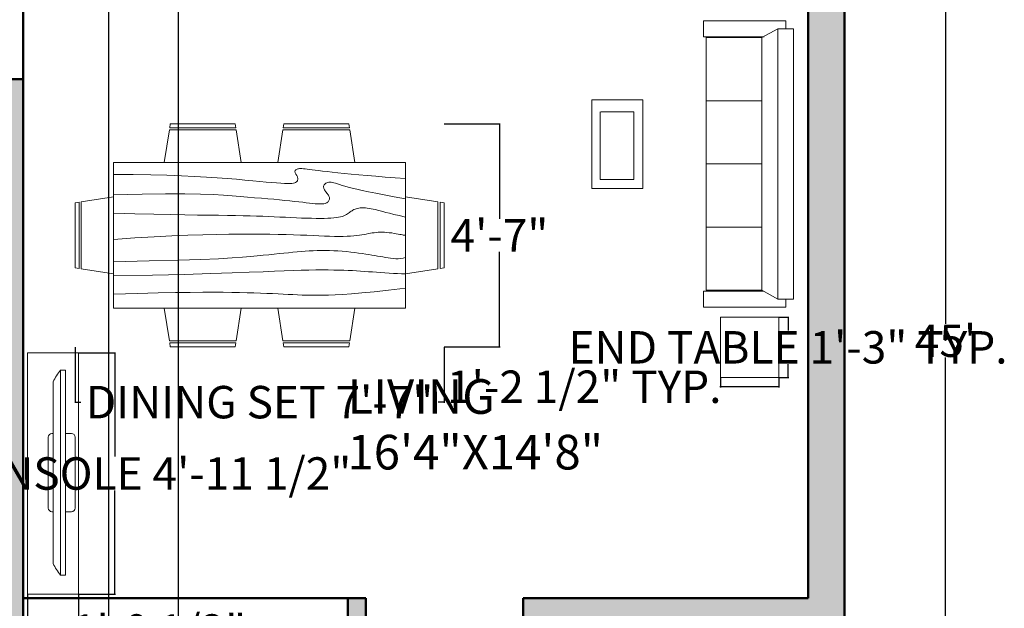
# Model space of a CAD drawing. Units: inches. Extents: x 22042254 to 25404563, y 17568978 to 17626777.
# Tile 42 of 45: x 22179940 to 22180183, y 17626402 to 17626547. Entities that reach past the tile are written whole.
import ezdxf

# ---------------------------------------------------------------- set-up
doc = ezdxf.new("R2010")
doc.units = ezdxf.units.IN
doc.header["$MEASUREMENT"] = 0
for name, color, linetype, lineweight in [('A-ANNO-DIMS', 2, 'Continuous', 18), ('A-AREA-IDEN', 7, 'Continuous', 18), ('A-WALL-PATT', 244, 'Continuous', 13), ('furniture', 8, 'Continuous', 18), ('walls', 252, 'Continuous', 50)]:
    doc.layers.add(name, color=color, linetype=linetype, lineweight=lineweight)
doc.styles.get("Standard").update_dxf_attribs({"font": 'arial.ttf'})
doc.dimstyles.get("Standard").update_dxf_attribs({"dimtxt": 8, "dimasz": 0.18, "dimexe": 0.18, "dimexo": 0.0625, "dimgap": 0.09, "dimtad": 0, "dimtih": 1, "dimtoh": 1, "dimzin": 0, "dimdsep": 46, "dimlunit": 3, "dimtxsty": 'Standard', "dimcen": 0.09, "dimadec": 0, "dimazin": 0, "dimtfac": 1, "dimtofl": 0, "dimtmove": 0, "dimatfit": 3, "dimfxl": 1, "dimtolj": 1, "dimtzin": 0, "dimarcsym": 0})

# ---------------------------------------------------------------- blocks, each defined once
blk = doc.blocks.new('*D2')
at = {"layer": 'A-ANNO-DIMS', "color": 0, "lineweight": -2, "transparency": 16777216}
for p, q in [((22180143.8, 17626737.78), (22180168.82, 17626737.78)), ((22180168.64, 17626737.6), (22180168.64, 17626471.94)), ((22180168.64, 17626197.96), (22180168.64, 17626463.62)), ((22180143.8, 17626197.78), (22180168.82, 17626197.78))]:
    blk.add_line(p, q, dxfattribs=at)
at = {"layer": 'A-ANNO-DIMS', "color": 0, "transparency": 16777216}
for points in [[(22180168.61, 17626737.6), (22180168.67, 17626737.6), (22180168.64, 17626737.78)], [(22180168.61, 17626197.96), (22180168.67, 17626197.96), (22180168.64, 17626197.78)]]:
    blk.add_solid(points, dxfattribs=at)
at = {"layer": 'Defpoints', "color": 0, "transparency": 16777216}
for p in [(22180143.73, 17626737.78), (22180168.64, 17626737.78), (22180143.73, 17626197.78)]:
    blk.add_point(p, dxfattribs=at)
at = {"layer": 'A-ANNO-DIMS', "color": 0, "transparency": 16777216, "insert": (22180168.64, 17626467.78), "char_height": 8, "attachment_point": 5}
blk.add_mtext("\\A1;45'", dxfattribs=at)
blk = doc.blocks.new('Dining Set - 36 x 72 in.')
for p, q in [((-22, 27.5), (-22.1562, 26.50042)), ((-22, 27.5), (-6, 27.5)), ((-5.8437, 26.49966), (-6, 27.5)), ((6, 27.5), (5.8438, 26.50042)), ((6, 27.5), (22, 27.5)), ((22.1563, 26.49966), (22, 27.5)), ((-22.2343, 26.00059), (-23.4847, 17.99762)), ((-22.2304, 26), (-5.7608, 26)), ((-5.8416, 26.5), (-22.1534, 26.5)), ((-4.5152, 17.99762), (-5.7655, 25.99926)), ((5.7657, 26.00059), (4.5153, 17.99762)), ((5.7696, 26), (22.2392, 26)), ((22.1584, 26.5), (5.8466, 26.5)), ((23.4848, 17.99762), (22.2345, 25.99926)), ((36, 18), (-36, 18)), ((-36, 18), (-36, -18)), ((36, -18), (36, 18)), ((-45.5, 8), (-44.5004, 8.15617)), ((-45.5, 8), (-45.5, -8)), ((-44.5, -8.15843), (-44.5, 8.15338)), ((-44.0006, 8.23428), (-35.9976, 9.48474)), ((-44, 8.23041), (-44, -8.23915)), ((44.0006, 8.23428), (35.9976, 9.48474)), ((44, 8.23041), (44, -8.23915)), ((44.5, -8.15843), (44.5, 8.15338)), ((45.5, 8), (44.5005, 8.15617)), ((45.5, 8), (45.5, -8)), ((-44.4997, -8.15631), (-45.5, -8)), ((-35.9976, -9.48476), (-43.9993, -8.2345)), ((35.9976, -9.48476), (43.9993, -8.2345)), ((44.4997, -8.15631), (45.5, -8)), ((-36, -18), (36, -18)), ((-22.2343, -26.0006), (-23.4847, -17.99762)), ((-4.5152, -17.99762), (-5.7655, -25.99928)), ((5.7657, -26.0006), (4.5153, -17.99762)), ((23.4848, -17.99762), (22.2345, -25.99928)), ((-22.2304, -26), (-5.7608, -26)), ((-22, -27.5), (-22.1562, -26.50044)), ((-5.8416, -26.5), (-22.1534, -26.5)), ((-5.8437, -26.49967), (-6, -27.5)), ((5.7696, -26), (22.2392, -26)), ((6, -27.5), (5.8438, -26.50044)), ((22.1584, -26.5), (5.8466, -26.5)), ((22.1563, -26.49967), (22, -27.5)), ((-22, -27.5), (-6, -27.5)), ((6, -27.5), (22, -27.5))]:
    blk.add_line(p, q)
for points in [[(-36, 15), (-31.1772, 14.97754), (-26.8079, 14.91406), (-22.8538, 14.81543), (-19.276, 14.6875), (-16.0362, 14.53613), (-13.0957, 14.36718), (-10.4159, 14.18652), (-7.9583, 14), (-5.6904, 13.81315), (-3.6035, 13.63021), (-1.6954, 13.45508), (0.0365, 13.29166), (1.5945, 13.14388), (2.9811, 13.01562), (4.1988, 12.9108), (5.25, 12.83333), (6.1393, 12.78613), (6.8802, 12.76823), (7.4883, 12.77767), (7.9792, 12.8125), (8.3685, 12.87077), (8.6719, 12.95052), (8.9049, 13.0498), (9.0833, 13.16666), (9.2205, 13.29899), (9.3216, 13.44401), (9.3895, 13.59879), (9.4271, 13.76041), (9.4373, 13.92594), (9.4232, 14.09245), (9.3875, 14.257), (9.3333, 14.41666), (9.2638, 14.56917), (9.1836, 14.71484), (9.0975, 14.85465), (9.0104, 14.98958), (8.9272, 15.1206), (8.8529, 15.2487), (8.7922, 15.37483), (8.75, 15.5), (8.7305, 15.62467), (8.7344, 15.74739), (8.7617, 15.86621), (8.8125, 15.97916), (8.8867, 16.08431), (8.9844, 16.17968), (9.1055, 16.26334), (9.25, 16.33333), (9.4189, 16.38802), (9.6172, 16.42708), (9.8506, 16.45052), (10.125, 16.45833), (10.4463, 16.45052), (10.8203, 16.42708), (11.2529, 16.38802), (11.75, 16.33333), (12.3184, 16.26318), (12.9694, 16.17838), (13.7151, 16.07991), (14.5677, 15.96875), (15.5395, 15.84586), (16.6426, 15.71224), (17.8893, 15.56884), (19.2917, 15.41666), (20.859, 15.25667), (22.5879, 15.08984), (24.4721, 14.91715), (26.5052, 14.73958), (28.6809, 14.5581), (30.9929, 14.3737), (33.4347, 14.18733), (36, 14)], [(-36, 10), (-28.9766, 10.14274), (-23.1725, 10.20442), (-18.4241, 10.19775), (-14.5677, 10.13541), (-11.4399, 10.03011), (-8.877, 9.89453), (-6.7154, 9.74137), (-4.7917, 9.58333), (-2.9698, 9.43082), (-1.2246, 9.28515), (0.4415, 9.14534), (2.026, 9.01041), (3.5266, 8.87939), (4.9408, 8.7513), (6.266, 8.62516), (7.5, 8.5), (8.6411, 8.37549), (9.6914, 8.2539), (10.6538, 8.13818), (11.5312, 8.03125), (12.3267, 7.93603), (13.043, 7.85547), (13.6831, 7.79248), (14.25, 7.75), (14.7471, 7.7303), (15.1797, 7.73307), (15.5537, 7.75732), (15.875, 7.80208), (16.1494, 7.86637), (16.3828, 7.94922), (16.5811, 8.04964), (16.75, 8.16666), (16.8944, 8.29915), (17.0143, 8.44531), (17.1089, 8.60319), (17.1771, 8.77083), (17.218, 8.94629), (17.2305, 9.1276), (17.2137, 9.31282), (17.1667, 9.5), (17.0895, 9.6875), (16.987, 9.875), (16.8649, 10.0625), (16.7292, 10.25), (16.5856, 10.4375), (16.4401, 10.625), (16.2985, 10.8125), (16.1667, 11), (16.05, 11.18733), (15.9518, 11.3737), (15.8752, 11.5581), (15.8229, 11.73958), (15.798, 11.91715), (15.8034, 12.08984), (15.842, 12.25667), (15.9167, 12.41666), (16.0295, 12.56836), (16.1784, 12.70833), (16.3605, 12.83268), (16.5729, 12.9375), (16.8127, 13.01888), (17.0768, 13.07291), (17.3625, 13.0957), (17.6667, 13.08333), (17.9894, 13.03312), (18.3418, 12.94726), (18.7382, 12.82918), (19.1927, 12.68229), (19.7195, 12.51001), (20.3327, 12.31575), (21.0465, 12.10294), (21.875, 11.875), (22.8357, 11.63354), (23.959, 11.37304), (25.2786, 11.08618), (26.8282, 10.76562), (28.6414, 10.40405), (30.752, 9.99414), (33.1936, 9.52856), (36, 9)], [(-36, 5.5), (-30.7157, 5.3348), (-26.069, 5.20963), (-21.9946, 5.11767), (-18.4271, 5.05208), (-15.3009, 5.00602), (-12.5508, 4.97265), (-10.1112, 4.94515), (-7.9167, 4.91666), (-5.909, 4.88167), (-4.0586, 4.83984), (-2.3429, 4.79215), (-0.7396, 4.73958), (0.7739, 4.6831), (2.22, 4.6237), (3.6213, 4.56233), (5, 4.5), (6.373, 4.43782), (7.7344, 4.3776), (9.0723, 4.32129), (10.375, 4.27083), (11.6309, 4.22819), (12.8281, 4.19531), (13.9551, 4.17415), (15, 4.16666), (15.954, 4.17448), (16.819, 4.19791), (17.6001, 4.23698), (18.3021, 4.29166), (18.9299, 4.36198), (19.4883, 4.44791), (19.9823, 4.54948), (20.4167, 4.66666), (20.7969, 4.79899), (21.1302, 4.94401), (21.4245, 5.09879), (21.6875, 5.26041), (21.9271, 5.42594), (22.1511, 5.59245), (22.3672, 5.757), (22.5834, 5.91666), (22.8065, 6.06868), (23.0404, 6.21093), (23.2879, 6.34147), (23.5521, 6.45833), (23.8358, 6.55957), (24.142, 6.64323), (24.4735, 6.70735), (24.8334, 6.75), (25.2235, 6.76969), (25.642, 6.76692), (26.0858, 6.74267), (26.5521, 6.69791), (27.0379, 6.63362), (27.5404, 6.55078), (28.0565, 6.45036), (28.5834, 6.33333), (29.1242, 6.19987), (29.7071, 6.04687), (30.3661, 5.87044), (31.1354, 5.66666), (32.0493, 5.43164), (33.142, 5.16146), (34.4475, 4.85221), (36, 4.5)], [(-36, -1), (-30.7915, -0.6591), (-26.0195, -0.38216), (-21.6519, -0.16284), (-17.6563, 0.00521), (-14.0005, 0.12833), (-10.6523, 0.21289), (-7.5796, 0.26522), (-4.75, 0.29166), (-2.134, 0.29793), (0.2878, 0.28711), (2.5317, 0.26163), (4.6146, 0.22396), (6.5529, 0.17651), (8.3633, 0.12174), (10.0623, 0.06209), (11.6667, 0), (13.1899, -0.06201), (14.6341, -0.1211), (15.9982, -0.17432), (17.2813, -0.21875), (18.4823, -0.25147), (19.6003, -0.26953), (20.6343, -0.27002), (21.5834, -0.25), (22.4481, -0.20768), (23.2357, -0.14584), (23.9549, -0.06836), (24.6146, 0.02083), (25.2235, 0.11784), (25.7904, 0.21875), (26.3241, 0.31966), (26.8334, 0.41666), (27.3265, 0.50618), (27.8099, 0.58593), (28.2894, 0.65397), (28.7709, 0.70833), (29.2601, 0.74707), (29.763, 0.76823), (30.2855, 0.76985), (30.8334, 0.75), (31.4088, 0.70784), (31.9994, 0.64713), (32.589, 0.57275), (33.1615, 0.48958), (33.7008, 0.4025), (34.1908, 0.3164), (34.6153, 0.23616), (34.9584, 0.16666), (35.2099, 0.11165), (35.3848, 0.07031), (35.504, 0.04069), (35.5886, 0.02083), (35.6594, 0.00879), (35.7377, 0.0026), (35.8442, 0.00032), (36, 0)], [(-36, -6.5), (-27.1843, -6.31267), (-20.084, -6.1263), (-14.469, -5.9419), (-10.1094, -5.76042), (-6.7752, -5.58285), (-4.2363, -5.41016), (-2.2629, -5.24333), (-0.625, -5.08334), (0.8708, -4.93099), (2.2715, -4.78646), (3.5872, -4.64974), (4.8281, -4.52084), (6.0046, -4.39974), (7.127, -4.28646), (8.2053, -4.18099), (9.25, -4.08334), (10.2705, -3.99382), (11.2734, -3.91407), (12.2647, -3.84603), (13.25, -3.79167), (14.2354, -3.75293), (15.2266, -3.73177), (16.2295, -3.73015), (17.25, -3.75), (18.2912, -3.79248), (19.3451, -3.85547), (20.4009, -3.93604), (21.4479, -4.03125), (22.4754, -4.13819), (23.4727, -4.25391), (24.4289, -4.37549), (25.3334, -4.5), (26.1785, -4.62492), (26.9694, -4.74935), (27.7145, -4.87281), (28.4219, -4.99479), (29.1, -5.11483), (29.7572, -5.23242), (30.4016, -5.34709), (31.0417, -5.45834), (31.6837, -5.56437), (32.3262, -5.65821), (32.9658, -5.73153), (33.599, -5.77604), (34.2224, -5.78345), (34.8327, -5.74545), (35.4264, -5.65373), (36, -5.5)], [(-36, -10), (-26.4022, -9.81299), (-18.4675, -9.62891), (-11.9839, -9.45069), (-6.7396, -9.28125), (-2.5226, -9.12354), (0.8789, -8.98047), (3.6769, -8.85498), (6.0833, -8.75), (8.2767, -8.66765), (10.3021, -8.60677), (12.1712, -8.56543), (13.8958, -8.54167), (15.4876, -8.53353), (16.9583, -8.53907), (18.3197, -8.55632), (19.5834, -8.58334), (20.7616, -8.61841), (21.8685, -8.66081), (22.9188, -8.71004), (23.9271, -8.76563), (24.9081, -8.82707), (25.8763, -8.89388), (26.8465, -8.96558), (27.8334, -9.04167), (28.8474, -9.12118), (29.8828, -9.20117), (30.93, -9.27824), (31.9792, -9.34896), (33.0205, -9.40991), (34.0443, -9.45768), (35.0407, -9.48885), (36, -9.5)], [(-36, -14.5), (-30.0881, -14.33513), (-25.0332, -14.21224), (-20.7312, -14.12647), (-17.0781, -14.07292), (-13.97, -14.04671), (-11.3027, -14.04297), (-8.9724, -14.05681), (-6.875, -14.08334), (-4.9224, -14.11833), (-3.0905, -14.16016), (-1.3709, -14.20785), (0.2448, -14.26042), (1.7647, -14.3169), (3.1973, -14.3763), (4.5507, -14.43767), (5.8333, -14.5), (7.0554, -14.5621), (8.235, -14.62175), (9.3922, -14.67652), (10.5469, -14.72396), (11.7192, -14.76164), (12.929, -14.78711), (14.1965, -14.79794), (15.5417, -14.79167), (16.9933, -14.76424), (18.6152, -14.70508), (20.4804, -14.60197), (22.6615, -14.44271), (25.2312, -14.21509), (28.2624, -13.9069), (31.8277, -13.50594), (36, -13)]]:
    blk.add_lwpolyline(points)
blk = doc.blocks.new('FABRIC SOFA 4S')
at = {"layer": 'furniture'}
for p, q in [((3, 54), (34, 54)), ((3, 51), (3, 54)), ((34, 48), (34, 54)), ((0, -51), (0, 51)), ((6, 51), (0, 51)), ((6, -51), (6, 51)), ((12, 47.63), (6, 51)), ((11.14, 48), (34, 48)), ((33, 23.81), (12, 23.81)), ((33, 0), (12, 0)), ((33, -23.81), (12, -23.81)), ((6, -51), (12, -47.63)), ((11.54, -48), (34, -48)), ((34, -48), (34, -54)), ((6, -51), (0, -51)), ((3, -54), (3, -51)), ((3, -54), (34, -54))]:
    blk.add_line(p, q, dxfattribs=at)
blk.add_lwpolyline([(12, -47.63), (12, 47.63), (33, 47.63), (33, -47.63)], close=True, dxfattribs=at)
blk = doc.blocks.new('PLASMA-LARGE')
at = {"layer": 'furniture'}
for p, q in [((-7.26, 0), (7.26, 0)), ((-18.61, -1), (18.61, -1)), ((-8, -1), (-8, -0.74)), ((8, -1), (8, -0.74)), ((-21, -2.5), (21, -2.5)), ((-21, -2.5), (-21, -3.5)), ((-21, -3.5), (21, -3.5)), ((-8, -3.5), (-8, -4.76)), ((8, -3.5), (8, -4.76)), ((21, -2.5), (21, -3.5)), ((-7.26, -5.5), (7.26, -5.5))]:
    blk.add_line(p, q, dxfattribs=at)
for centre, radius, start, end in [((-7.26, -0.74), 0.744, 90, 180), ((7.26, -0.74), 0.744, 0, 90), ((-13.97, -11.05), 11.07, 114.7602, 129.4175), ((13.97, -11.05), 11.07, 50.5825, 65.2398), ((-7.26, -4.76), 0.744, 180, 270), ((7.26, -4.76), 0.744, 270, 0)]:
    blk.add_arc(centre, radius, start, end, dxfattribs=at)
blk = doc.blocks.new('TV-CONSOLE')
for p, q in [((8.99, 35.63), (-6.22, 35.63)), ((-6.22, 35.63), (-6.22, -36.14)), ((8.99, -36.14), (8.99, 35.63)), ((-6.22, -36.14), (8.99, -36.14))]:
    blk.add_line(p, q)
at = {"xscale": 1.450199298177205, "yscale": 1.450199298177205, "zscale": 1.450199298177205, "rotation": 90}
blk.add_blockref('PLASMA-LARGE', (0, 0), dxfattribs=at)
blk = doc.blocks.new('END-TABLE')
for p, q in [((0, 0), (0, 14.95)), ((0, 14.95), (14.41, 14.95)), ((14.41, 14.95), (14.41, 0)), ((0, 0), (14.41, 0))]:
    blk.add_line(p, q)
blk = doc.blocks.new('*D40')
at = {"layer": 'A-ANNO-DIMS', "color": 0, "lineweight": -2, "transparency": 16777216}
for p, q in [((22179954.93, 17626464.83), (22179963.98, 17626464.83)), ((22179963.8, 17626464.65), (22179963.8, 17626439.26)), ((22179963.8, 17626405.42), (22179963.8, 17626430.8)), ((22179954.93, 17626405.24), (22179963.98, 17626405.24))]:
    blk.add_line(p, q, dxfattribs=at)
at = {"layer": 'A-ANNO-DIMS', "color": 0, "transparency": 16777216}
for points in [[(22179963.77, 17626464.65), (22179963.83, 17626464.65), (22179963.8, 17626464.83)], [(22179963.77, 17626405.42), (22179963.83, 17626405.42), (22179963.8, 17626405.24)]]:
    blk.add_solid(points, dxfattribs=at)
at = {"layer": 'Defpoints', "color": 0, "transparency": 16777216}
for p in [(22179954.87, 17626464.83), (22179963.8, 17626464.83), (22179954.87, 17626405.24)]:
    blk.add_point(p, dxfattribs=at)
at = {"layer": 'A-ANNO-DIMS', "color": 0, "transparency": 16777216, "insert": (22179963.8, 17626435.03), "char_height": 8, "attachment_point": 5}
blk.add_mtext('\\A1;TV CONSOLE 4\'-11 1/2"', dxfattribs=at)
blk = doc.blocks.new('*D41')
at = {"layer": 'A-ANNO-DIMS', "color": 0, "lineweight": -2, "transparency": 16777216}
for p, q in [((22179942.23, 17626405.18), (22179942.23, 17626396.12)), ((22179954.87, 17626405.18), (22179954.87, 17626396.12)), ((22179942.41, 17626396.3), (22179954.69, 17626396.3)), ((22179954.87, 17626396.3), (22179955.05, 17626396.3))]:
    blk.add_line(p, q, dxfattribs=at)
at = {"layer": 'A-ANNO-DIMS', "color": 0, "transparency": 16777216}
for points in [[(22179942.41, 17626396.33), (22179942.41, 17626396.27), (22179942.23, 17626396.3)], [(22179954.69, 17626396.33), (22179954.69, 17626396.27), (22179954.87, 17626396.3)]]:
    blk.add_solid(points, dxfattribs=at)
at = {"layer": 'Defpoints', "color": 0, "transparency": 16777216}
for p in [(22179942.23, 17626405.24), (22179954.87, 17626405.24), (22179954.87, 17626396.3)]:
    blk.add_point(p, dxfattribs=at)
at = {"layer": 'A-ANNO-DIMS', "color": 0, "transparency": 16777216, "insert": (22179974.71, 17626396.3), "char_height": 8, "attachment_point": 5}
blk.add_mtext('\\A1;1\'-0 1/2"', dxfattribs=at)
blk = doc.blocks.new('*D50')
at = {"layer": 'A-ANNO-DIMS', "color": 0, "lineweight": -2, "transparency": 16777216}
for p, q in [((22180127.63, 17626473.62), (22180129.99, 17626473.62)), ((22180129.81, 17626473.44), (22180129.81, 17626470.33)), ((22180129.81, 17626458.86), (22180129.81, 17626461.97)), ((22180127.63, 17626458.68), (22180129.99, 17626458.68))]:
    blk.add_line(p, q, dxfattribs=at)
at = {"layer": 'A-ANNO-DIMS', "color": 0, "transparency": 16777216}
for points in [[(22180129.78, 17626473.44), (22180129.84, 17626473.44), (22180129.81, 17626473.62)], [(22180129.78, 17626458.86), (22180129.84, 17626458.86), (22180129.81, 17626458.68)]]:
    blk.add_solid(points, dxfattribs=at)
at = {"layer": 'Defpoints', "color": 0, "transparency": 16777216}
for p in [(22180127.57, 17626473.62), (22180127.57, 17626458.68), (22180129.81, 17626458.68)]:
    blk.add_point(p, dxfattribs=at)
at = {"layer": 'A-ANNO-DIMS', "color": 0, "transparency": 16777216, "insert": (22180129.81, 17626466.15), "char_height": 8, "attachment_point": 5}
blk.add_mtext('\\A1;END TABLE 1\'-3" TYP.', dxfattribs=at)
blk = doc.blocks.new('*D51')
at = {"layer": 'A-ANNO-DIMS', "color": 0, "lineweight": -2, "transparency": 16777216}
for p, q in [((22180113.16, 17626458.61), (22180113.16, 17626456.25)), ((22180127.57, 17626458.61), (22180127.57, 17626456.25)), ((22180113.16, 17626456.43), (22180112.98, 17626456.43)), ((22180127.39, 17626456.43), (22180113.34, 17626456.43))]:
    blk.add_line(p, q, dxfattribs=at)
at = {"layer": 'A-ANNO-DIMS', "color": 0, "transparency": 16777216}
for points in [[(22180113.34, 17626456.46), (22180113.34, 17626456.4), (22180113.16, 17626456.43)], [(22180127.39, 17626456.46), (22180127.39, 17626456.4), (22180127.57, 17626456.43)]]:
    blk.add_solid(points, dxfattribs=at)
at = {"layer": 'Defpoints', "color": 0, "transparency": 16777216}
for p in [(22180113.16, 17626458.68), (22180127.57, 17626458.68), (22180113.16, 17626456.43)]:
    blk.add_point(p, dxfattribs=at)
at = {"layer": 'A-ANNO-DIMS', "color": 0, "transparency": 16777216, "insert": (22180079.56, 17626456.43), "char_height": 8, "attachment_point": 5}
blk.add_mtext('\\A1;1\'-2 1/2" TYP.', dxfattribs=at)
blk = doc.blocks.new('*D52')
at = {"layer": 'A-ANNO-DIMS', "color": 0, "lineweight": -2, "transparency": 16777216}
for p, q in [((22179953.99, 17626466.22), (22179953.99, 17626452.45)), ((22180044.99, 17626466.22), (22180044.99, 17626452.45)), ((22179954.17, 17626452.63), (22179955.43, 17626452.63)), ((22180044.81, 17626452.63), (22180043.54, 17626452.63))]:
    blk.add_line(p, q, dxfattribs=at)
at = {"layer": 'A-ANNO-DIMS', "color": 0, "transparency": 16777216}
for points in [[(22179954.17, 17626452.66), (22179954.17, 17626452.6), (22179953.99, 17626452.63)], [(22180044.81, 17626452.66), (22180044.81, 17626452.6), (22180044.99, 17626452.63)]]:
    blk.add_solid(points, dxfattribs=at)
at = {"layer": 'Defpoints', "color": 0, "transparency": 16777216}
for p in [(22179953.99, 17626466.28), (22180044.99, 17626466.28), (22180044.99, 17626452.63)]:
    blk.add_point(p, dxfattribs=at)
at = {"layer": 'A-ANNO-DIMS', "color": 0, "transparency": 16777216, "insert": (22179999.49, 17626452.63), "char_height": 8, "attachment_point": 5}
blk.add_mtext('\\A1;DINING SET 7\'-7"', dxfattribs=at)
blk = doc.blocks.new('*D53')
at = {"layer": 'A-ANNO-DIMS', "color": 0, "lineweight": -2, "transparency": 16777216}
for p, q in [((22180045.05, 17626521.28), (22180058.82, 17626521.28)), ((22180058.64, 17626521.1), (22180058.64, 17626497.87)), ((22180058.64, 17626466.46), (22180058.64, 17626489.69)), ((22180045.05, 17626466.28), (22180058.82, 17626466.28))]:
    blk.add_line(p, q, dxfattribs=at)
at = {"layer": 'A-ANNO-DIMS', "color": 0, "transparency": 16777216}
for points in [[(22180058.61, 17626521.1), (22180058.67, 17626521.1), (22180058.64, 17626521.28)], [(22180058.61, 17626466.46), (22180058.67, 17626466.46), (22180058.64, 17626466.28)]]:
    blk.add_solid(points, dxfattribs=at)
at = {"layer": 'Defpoints', "color": 0, "transparency": 16777216}
for p in [(22180044.99, 17626521.28), (22180058.64, 17626521.28), (22180044.99, 17626466.28)]:
    blk.add_point(p, dxfattribs=at)
at = {"layer": 'A-ANNO-DIMS', "color": 0, "transparency": 16777216, "insert": (22180058.64, 17626493.78), "char_height": 8, "attachment_point": 5}
blk.add_mtext('\\A1;4\'-7"', dxfattribs=at)
blk = doc.blocks.new('*D63')
at = {"layer": 'A-ANNO-DIMS', "color": 0, "lineweight": -2, "transparency": 16777216}
for p, q in [((22179962.22, 17626655.72), (22179962.22, 17626158.2)), ((22179979.38, 17626655.72), (22179979.38, 17626158.2)), ((22179962.4, 17626158.38), (22179979.2, 17626158.38)), ((22179979.38, 17626158.38), (22179979.56, 17626158.38))]:
    blk.add_line(p, q, dxfattribs=at)
at = {"layer": 'A-ANNO-DIMS', "color": 0, "transparency": 16777216}
for points in [[(22179962.4, 17626158.41), (22179962.4, 17626158.35), (22179962.22, 17626158.38)], [(22179979.2, 17626158.41), (22179979.2, 17626158.35), (22179979.38, 17626158.38)]]:
    blk.add_solid(points, dxfattribs=at)
at = {"layer": 'Defpoints', "color": 0, "transparency": 16777216}
for p in [(22179962.22, 17626655.78), (22179979.38, 17626655.78), (22179979.38, 17626158.38)]:
    blk.add_point(p, dxfattribs=at)
at = {"layer": 'A-ANNO-DIMS', "color": 0, "transparency": 16777216, "insert": (22179989.91, 17626158.38), "char_height": 8, "attachment_point": 5}
blk.add_mtext('\\A1;1\'-5"', dxfattribs=at)

msp = doc.modelspace()

# ---------------------------------------------------------------- hatches: boundary and pattern name
at = {"layer": 'A-WALL-PATT'}
h = msp.add_hatch(color=256, dxfattribs=at)
h.dxf.hatch_style = 1
h.paths.add_polyline_path([(22179792.734, 17626580.28), (22179888.734, 17626580.28), (22179888.734, 17626559.623), (22179893.234, 17626559.623), (22179893.234, 17626580.28), (22179900.438, 17626580.28), (22179900.438, 17626584.78), (22179792.734, 17626584.78), (22179792.734, 17626728.78), (22180134.734, 17626728.78), (22180134.734, 17626584.78), (22180035.602, 17626584.78), (22180004.432, 17626584.78), (22180001.734, 17626584.78), (22180001.734, 17626580.28), (22180134.734, 17626580.28), (22180134.734, 17626404.28), (22180064.487, 17626404.28), (22180064.487, 17626399.78), (22180134.734, 17626399.78), (22180134.734, 17626197.78), (22180143.734, 17626197.78), (22180143.734, 17626737.78), (22179783.734, 17626737.78), (22179783.734, 17626197.78), (22179792.734, 17626197.78), (22179792.734, 17626394.78), (22179936.734, 17626394.78), (22179936.734, 17626383.208), (22179941.234, 17626383.208), (22179941.234, 17626532.28), (22179927.066, 17626532.28), (22179927.066, 17626527.78), (22179928.072, 17626527.78), (22179936.734, 17626527.78), (22179936.734, 17626403.78), (22179792.734, 17626403.78), (22179792.734, 17626527.78), (22179905.094, 17626527.78), (22179905.094, 17626532.28), (22179792.734, 17626532.28)])
h = msp.add_hatch(color=256, dxfattribs=at)
h.dxf.hatch_style = 1
h.paths.add_polyline_path([(22179941.234, 17626336.599), (22179936.734, 17626336.599), (22179936.734, 17626270.28), (22180065.734, 17626270.28), (22180065.734, 17626197.78), (22180074.734, 17626197.78), (22180074.734, 17626279.28), (22180025.734, 17626279.28), (22180025.734, 17626404.28), (22180021.234, 17626404.28), (22180021.234, 17626279.28), (22179941.234, 17626279.28), (22179941.234, 17626327.28), (22179991.805, 17626327.28), (22179991.805, 17626331.78), (22179941.234, 17626331.78)])
h.paths.add_polyline_path([(22180036.005, 17626206.78), (22179936.734, 17626206.78), (22179936.734, 17626197.78), (22180036.005, 17626197.78)], flags=17)
h.paths.add_polyline_path([(22179836.995, 17626451.976), (22179902.189, 17626451.976), (22179902.189, 17626465.064), (22179836.995, 17626465.064)], flags=9)
h.paths.add_polyline_path([(22179836.966, 17626465.674), (22179903.069, 17626465.674), (22179903.069, 17626478.937), (22179836.966, 17626478.937)], flags=9)
h.paths.add_polyline_path([(22180055.036, 17626649.533), (22180120.23, 17626649.533), (22180120.23, 17626662.622), (22180055.036, 17626662.622)], flags=9)
h.paths.add_polyline_path([(22180055.007, 17626663.231), (22180121.111, 17626663.231), (22180121.111, 17626676.495), (22180055.007, 17626676.495)], flags=9)

# ---------------------------------------------------------------- linework, layer by layer
at = {"layer": 'furniture'}
for p, q in [((22180081.463, 17626505.363), (22180081.463, 17626527.179)), ((22180081.463, 17626527.179), (22180093.976, 17626527.179)), ((22180081.463, 17626527.179), (22180081.463, 17626505.363)), ((22180093.976, 17626527.179), (22180081.463, 17626527.179)), ((22180093.976, 17626527.179), (22180093.976, 17626505.363)), ((22180093.976, 17626505.363), (22180093.976, 17626527.179)), ((22180083.454, 17626507.533), (22180083.454, 17626524.238)), ((22180083.656, 17626524.238), (22180091.815, 17626524.238)), ((22180091.815, 17626524.238), (22180091.815, 17626507.533)), ((22180091.815, 17626507.533), (22180083.454, 17626507.533)), ((22180093.976, 17626505.363), (22180081.463, 17626505.363)), ((22180081.463, 17626505.363), (22180093.976, 17626505.363))]:
    msp.add_line(p, q, dxfattribs=at)
at = {"layer": 'walls'}
for p, q in [((22180143.734, 17626737.78), (22180143.734, 17626197.78)), ((22179941.234, 17626532.28), (22179941.234, 17626580.28)), ((22180134.734, 17626580.28), (22180134.734, 17626404.28)), ((22179792.734, 17626532.28), (22179941.234, 17626532.28)), ((22179941.234, 17626383.208), (22179941.234, 17626532.28)), ((22179941.234, 17626404.28), (22180025.734, 17626404.28)), ((22180021.234, 17626279.28), (22180021.234, 17626404.28)), ((22180025.734, 17626279.28), (22180025.734, 17626404.28)), ((22180064.487, 17626404.28), (22180064.487, 17626399.78)), ((22180064.487, 17626404.28), (22180134.734, 17626404.28))]:
    msp.add_line(p, q, dxfattribs=at)

# ---------------------------------------------------------------- block references
at = {"layer": 'furniture', "xscale": -0.6537939928824033, "yscale": 0.6537939928824033, "zscale": 0.6537939928824033, "rotation": 359.9999999998932}
msp.add_blockref('FABRIC SOFA 4S', (22180131.188, 17626511.392), dxfattribs=at)
at = {"layer": 'furniture'}
msp.add_blockref('Dining Set - 36 x 72 in.', (22179999.487, 17626493.778), dxfattribs=at)
at = {"layer": 'furniture', "rotation": 180}
msp.add_blockref('END-TABLE', (22180127.568, 17626473.621), dxfattribs=at)
at = {"layer": 'furniture', "xscale": 0.8303208636481411, "yscale": 0.8303208636481411}
msp.add_blockref('TV-CONSOLE', (22179947.399, 17626435.243), dxfattribs=at)

# ---------------------------------------------------------------- texts
at = {"layer": 'A-AREA-IDEN'}
for s, height, p in [('LIVING', 8.5453, (22180021.174, 17626449.75)), ('16\'4"X14\'8"', 8.54529, (22180021.174, 17626436.022))]:
    msp.add_text(s, height=height, dxfattribs=at).set_placement(p)

# ---------------------------------------------------------------- dimensions: what is measured, and where the dimension line sits
at = {"layer": 'A-ANNO-DIMS'}
for base, p1, p2, override, picture, middle in [((22180168.64, 17626737.78), (22180143.734, 17626197.78), (22180143.734, 17626737.78), {"dimclrd": 0, "dimclre": 0, "dimclrt": 0}, '*D2', (22180168.64, 17626467.78)), ((22180058.637, 17626521.278), (22180044.987, 17626466.278), (22180044.987, 17626521.278), {"dimdec": 1, "dimlfac": 1, "dimrnd": 0, "dimzin": 1, "dimdsep": 46, "dimlunit": 4, "dimfrac": 2}, '*D53', (22180058.637, 17626493.778))]:
    dim = msp.add_linear_dim(base=base, p1=p1, p2=p2, angle=90, dimstyle='Standard', override=override, dxfattribs=at)
    dim.commit()
    dim.dimension.update_dxf_attribs({"geometry": picture, "text_midpoint": middle})
for base, p1, p2, picture, middle in [((22179979.384, 17626158.384), (22179962.224, 17626655.782), (22179979.384, 17626655.782), '*D63', (22179989.911, 17626158.384)), ((22179954.866, 17626396.301), (22179942.234, 17626405.239), (22179954.866, 17626405.239), '*D41', (22179974.713, 17626396.301))]:
    dim = msp.add_linear_dim(base=base, p1=p1, p2=p2, dimstyle='Standard', override={"dimdec": 1, "dimlfac": 1, "dimrnd": 0, "dimzin": 1, "dimdsep": 46, "dimlunit": 4, "dimfrac": 2}, dxfattribs=at)
    dim.commit()
    dim.dimension.update_dxf_attribs({"geometry": picture, "text_midpoint": middle})
for base, p1, p2, angle, text, picture, middle in [((22180129.81, 17626458.675), (22180127.568, 17626473.621), (22180127.568, 17626458.675), 270, 'END TABLE <> TYP.', '*D50', (22180129.81, 17626466.148)), ((22180113.158, 17626456.434), (22180127.568, 17626458.675), (22180113.158, 17626458.675), 180, '<> TYP.', '*D51', (22180079.562, 17626456.434)), ((22179963.805, 17626464.828), (22179954.866, 17626405.239), (22179954.866, 17626464.828), 90, 'TV CONSOLE <>', '*D40', (22179963.805, 17626435.034))]:
    dim = msp.add_linear_dim(base=base, p1=p1, p2=p2, angle=angle, text=text, dimstyle='Standard', override={"dimdec": 1, "dimlfac": 1, "dimrnd": 0, "dimzin": 1, "dimdsep": 46, "dimlunit": 4, "dimfrac": 2}, dxfattribs=at)
    dim.commit()
    dim.dimension.update_dxf_attribs({"geometry": picture, "text_midpoint": middle})
dim = msp.add_linear_dim(base=(22180044.987, 17626452.628), p1=(22179953.987, 17626466.278), p2=(22180044.987, 17626466.278), text='DINING SET <>', dimstyle='Standard', override={"dimdec": 1, "dimlfac": 1, "dimrnd": 0, "dimzin": 1, "dimdsep": 46, "dimlunit": 4, "dimfrac": 2}, dxfattribs=at)
dim.commit()
dim.dimension.update_dxf_attribs({"geometry": '*D52', "text_midpoint": (22179999.487, 17626452.628)})

doc.saveas('drawing.dxf')
